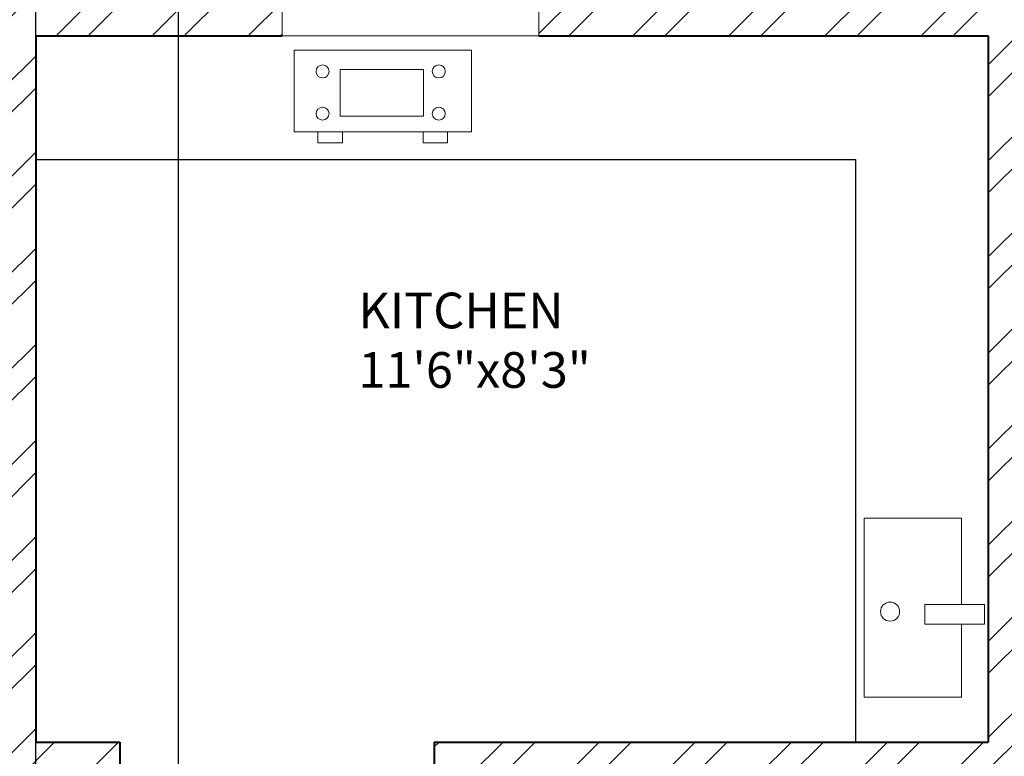
# Model space of a CAD drawing. Units: inches. Extents: x 1601 to 2297, y 1496 to 2631.
# Tile 55 of 57: x 2033 to 2171, y 2422 to 2526. Entities that reach past the tile are written whole.
import ezdxf

# ---------------------------------------------------------------- set-up
doc = ezdxf.new("R2010")
doc.units = ezdxf.units.IN
for name, color, linetype, lineweight in [('A-ANNO-DIMS', 2, 'Continuous', 18), ('A-AREA-IDEN', 7, 'Continuous', 18), ('A-EQPM', 8, 'Continuous', 18), ('A-FLOR-CASE', 8, 'Continuous', 25), ('A-FLOR-FIXT', 9, 'Continuous', 20), ('A-GLAZ', 161, 'Continuous', 20), ('A-WALL', 7, 'Continuous', 40), ('A-WALL-PATT', 215, 'Continuous', 13)]:
    doc.layers.add(name, color=color, linetype=linetype, lineweight=lineweight)
doc.styles.get("Standard").update_dxf_attribs({"font": 'arial.ttf'})
doc.dimstyles.get("Standard").update_dxf_attribs({"dimtxt": 0.18, "dimasz": 0.18, "dimexe": 0.18, "dimexo": 0.0625, "dimgap": 0.09, "dimtad": 0, "dimtih": 1, "dimtoh": 1, "dimdec": 4, "dimzin": 0, "dimdsep": 46, "dimtxsty": 'Standard', "dimcen": 0.09, "dimadec": 0, "dimazin": 0, "dimtfac": 1, "dimtdec": 4, "dimtofl": 0, "dimtmove": 0, "dimatfit": 3, "dimfxl": 1, "dimtolj": 1, "dimtzin": 0, "dimarcsym": 0})

# ---------------------------------------------------------------- blocks, each defined once
blk = doc.blocks.new('COOKTOP-4-BURNER')
for points in [[(0, 12.95), (24.89, 12.95), (24.89, 1.51), (0, 1.51)], [(6.45, 10.25), (18.15, 10.25), (18.15, 3.74), (6.45, 3.74)], [(3.35, 1.51), (6.77, 1.51), (6.77, 0), (3.35, 0)], [(18.09, 1.51), (21.52, 1.51), (21.52, 0), (18.09, 0)], [(18.09, 1.51), (21.52, 1.51), (21.52, 0), (18.09, 0)]]:
    blk.add_lwpolyline(points, close=True)
for centre in [(4, 9.99), (20.29, 9.99), (4, 4.07), (20.29, 4.07)]:
    blk.add_circle(centre, 0.91)
blk = doc.blocks.new('SINK-KITCHEN')
blk.add_lwpolyline([(13.62, 10.25), (13.62, 0), (0, 0), (0, 25.08), (13.62, 25.08), (13.62, 13.01)])
blk.add_lwpolyline([(8.47, 13.01), (16.82, 13.01), (16.82, 10.25), (8.47, 10.25)], close=True)
blk.add_circle((3.61, 11.99), 1.34)
blk = doc.blocks.new('*D40')
at = {"layer": 'A-ANNO-DIMS', "color": 0, "lineweight": -2, "transparency": 16777216}
for p, q in [((2035.54, 1986.39), (2035.54, 2581.06)), ((2035.72, 2580.88), (2045.08, 2580.88)), ((2055.37, 2580.88), (2046.01, 2580.88)), ((2055.55, 1986.39), (2055.55, 2581.06))]:
    blk.add_line(p, q, dxfattribs=at)
at = {"layer": 'A-ANNO-DIMS', "color": 0, "transparency": 16777216}
for points in [[(2035.72, 2580.91), (2035.72, 2580.85), (2035.54, 2580.88)], [(2055.37, 2580.91), (2055.37, 2580.85), (2055.55, 2580.88)]]:
    blk.add_solid(points, dxfattribs=at)
at = {"layer": 'Defpoints', "color": 0, "transparency": 16777216}
for p in [(2055.55, 2580.88), (2035.54, 1986.33), (2055.55, 1986.33)]:
    blk.add_point(p, dxfattribs=at)
at = {"layer": 'A-ANNO-DIMS', "color": 0, "transparency": 16777216, "insert": (2045.54, 2580.88), "char_height": 0.18, "attachment_point": 5}
blk.add_mtext('\\A1;20.014', dxfattribs=at)

msp = doc.modelspace()

# ---------------------------------------------------------------- hatches: boundary and pattern name
at = {"layer": 'A-WALL-PATT'}
h = msp.add_hatch(dxfattribs=at)
h.set_pattern_fill('ANSI32', color=256)
h.paths.add_polyline_path([(1842.0336, 2528.0767), (1842.0336, 2532.3254), (1686.0373, 2532.3254), (1686.0373, 2492.9493), (1695.0373, 2492.9493), (1695.0373, 2523.3254), (1827.0373, 2523.3254), (1827.0373, 2416.8254), (1834.6225, 2416.8254), (1834.6225, 2419.0754), (1834.6225, 2421.3254), (1831.5373, 2421.3254), (1831.5373, 2523.3254), (1842.0336, 2523.3254)])
h.paths.add_polyline_path([(1695.0373, 2432.9493), (1686.0373, 2432.9493), (1686.0373, 2325.989), (1695.0373, 2325.989), (1695.0373, 2347.8254), (1827.0373, 2347.8254), (1827.0373, 2287.8254), (1823.2991, 2287.8254), (1823.2991, 2283.3254), (1847.9422, 2283.3254), (1847.9422, 2285.5754), (1847.9422, 2287.8254), (1831.5373, 2287.8254), (1831.5373, 2347.8254), (1846.9946, 2347.8254), (1846.9946, 2350.0754), (1846.9946, 2352.3254), (1695.0373, 2352.3254)])
h.paths.add_polyline_path([(1807.1169, 1573.5395), (2055.0405, 1573.5395), (2055.0405, 1610.6322), (1807.1169, 1610.6322)], flags=9)
h.paths.add_polyline_path([(1841.1631, 1712.7967), (1870.3957, 1712.7967), (1870.3957, 1731.454), (1841.1631, 1731.454)], flags=9)
h.paths.add_polyline_path([(2144.3862, 1772.185), (2191.0233, 1772.185), (2191.0233, 1790.8423), (2144.3862, 1790.8423)], flags=9)
h.paths.add_polyline_path([(2143.0128, 1827.3312), (2177.9958, 1827.3312), (2177.9958, 1845.9886), (2143.0128, 1845.9886)], flags=9)
h.paths.add_polyline_path([(2041.2439, 1833.5691), (2070.8516, 1833.5691), (2070.8516, 1852.2264), (2041.2439, 1852.2264)], flags=9)
h.paths.add_polyline_path([(2097.2791, 1947.0598), (2134.2061, 1947.0598), (2134.2061, 1965.7171), (2097.2791, 1965.7171)], flags=9)
h.paths.add_polyline_path([(2214.995, 1904.3124), (2214.995, 1942.2899), (2196.3376, 1942.2899), (2196.3376, 1904.3124)], flags=9)
h.paths.add_polyline_path([(2186.6284, 2043.8031), (2219.7935, 2043.8031), (2219.7935, 2062.4605), (2186.6284, 2062.4605)], flags=9)
h.paths.add_polyline_path([(2064.0877, 2031.616), (2097.4949, 2031.616), (2097.4949, 2050.2734), (2064.0877, 2050.2734)], flags=9)
h.paths.add_polyline_path([(1973.1349, 1986.0688), (2008.4009, 1986.0688), (2008.4009, 2004.7261), (1973.1349, 2004.7261)], flags=9)
h.paths.add_polyline_path([(1976.3676, 2106.9635), (2005.7469, 2106.9635), (2005.7469, 2125.6209), (1976.3676, 2125.6209)], flags=9)
h.paths.add_polyline_path([(1991.7852, 2180.4863), (2027.0513, 2180.4863), (2027.0513, 2199.1437), (1991.7852, 2199.1437)], flags=9)
h.paths.add_polyline_path([(2106.1801, 2187.9359), (2152.2101, 2187.9359), (2152.2101, 2206.5932), (2106.1801, 2206.5932)], flags=9)
h.paths.add_polyline_path([(2148.6686, 2262.2542), (2182.318, 2262.2542), (2182.318, 2280.9115), (2148.6686, 2280.9115)], flags=9)
h.paths.add_polyline_path([(2041.6327, 2252.8147), (2071.2405, 2252.8147), (2071.2405, 2271.4721), (2041.6327, 2271.4721)], flags=9)
h.paths.add_polyline_path([(2063.9734, 2375.4265), (2100.9004, 2375.4265), (2100.9004, 2394.0839), (2063.9734, 2394.0839)], flags=9)
h.paths.add_polyline_path([(2216.4955, 2330.9748), (2216.4955, 2370.2654), (2197.8381, 2370.2654), (2197.8381, 2330.9748)], flags=9)
h.paths.add_polyline_path([(2179.1416, 2485.8687), (2212.3067, 2485.8687), (2212.3067, 2504.5261), (2179.1416, 2504.5261)], flags=9)
h.paths.add_polyline_path([(2078.7442, 2471.1516), (2112.1514, 2471.1516), (2112.1514, 2489.809), (2078.7442, 2489.809)], flags=9)
h.paths.add_polyline_path([(1915.9631, 2329.4668), (1952.8902, 2329.4668), (1952.8902, 2348.1241), (1915.9631, 2348.1241)], flags=9)
h.paths.add_polyline_path([(1904.3189, 2499.6709), (1940.4512, 2499.6709), (1940.4512, 2518.3282), (1904.3189, 2518.3282)], flags=9)
h.paths.add_polyline_path([(1892.3665, 2100.4595), (1925.6374, 2100.4595), (1925.6374, 2119.1169), (1892.3665, 2119.1169)], flags=9)
h.paths.add_polyline_path([(1909.2984, 1805.9631), (1946.2254, 1805.9631), (1946.2254, 1824.6205), (1909.2984, 1824.6205)], flags=9)
h.paths.add_polyline_path([(1934.6056, 1658.616), (1970.738, 1658.616), (1970.738, 1677.2733), (1934.6056, 1677.2733)], flags=9)
h.paths.add_polyline_path([(1711.2052, 1789.8902), (1750.0456, 1789.8902), (1750.0456, 1808.5476), (1711.2052, 1808.5476)], flags=9)
h.paths.add_polyline_path([(1742.7874, 1854.6743), (1771.9449, 1854.6743), (1771.9449, 1873.3317), (1742.7874, 1873.3317)], flags=9)
h.paths.add_polyline_path([(1807.3592, 1997.7912), (1850.1116, 1997.7912), (1850.1116, 2016.4486), (1807.3592, 2016.4486)], flags=9)
h.paths.add_polyline_path([(1717.4579, 2237.7844), (1760.2103, 2237.7844), (1760.2103, 2256.4417), (1717.4579, 2256.4417)], flags=9)
h.paths.add_polyline_path([(1780.9285, 2324.0623), (1810.086, 2324.0623), (1810.086, 2342.7197), (1780.9285, 2342.7197)], flags=25)
h.paths.add_polyline_path([(1837.696, 2449.2024), (1866.9286, 2449.2024), (1866.9286, 2467.8598), (1837.696, 2467.8598)], flags=9)
h.paths.add_polyline_path([(1712.7752, 2484.9404), (1751.6156, 2484.9404), (1751.6156, 2503.5977), (1712.7752, 2503.5977)], flags=25)
h = msp.add_hatch(dxfattribs=at)
h.set_pattern_fill('ANSI32', color=256)
h.paths.add_polyline_path([(2230.5373, 2532.3254), (2106.0595, 2532.3254), (2106.0595, 2523.3254), (2169.0373, 2523.3254), (2169.0373, 2424.3254), (2091.3989, 2424.3254), (2091.3989, 2419.8254), (2169.0373, 2419.8254), (2169.0373, 2408.1385), (2178.0373, 2408.1385), (2178.0373, 2419.8254), (2181.0581, 2419.8254), (2181.0581, 2422.0754), (2181.0581, 2424.3254), (2178.0373, 2424.3254), (2178.0373, 2523.3254), (2226.0373, 2523.3254), (2226.0373, 2424.3254), (2206.6251, 2424.3254), (2206.6251, 2419.8254), (2226.0373, 2419.8254), (2226.0373, 2299.8254), (2226.0373, 2295.3254), (2178.0373, 2295.3254), (2178.0373, 2312.1385), (2169.0373, 2312.1385), (2169.0373, 2295.3254), (2130.0373, 2295.3254), (2130.0373, 2279.1364), (2128.0593, 2279.1364), (2128.0593, 2274.6364), (2130.0373, 2274.6364), (2130.0373, 2260.7505), (2134.5373, 2260.7505), (2134.5373, 2290.8254), (2226.0373, 2290.8254), (2226.0373, 2279.2475), (2230.5373, 2279.2475), (2230.5373, 2347.8254)])
h.paths.add_polyline_path([(2070.0595, 2532.3254), (2031.0373, 2532.3254), (2031.0373, 2466.3254), (2003.9878, 2466.3254), (2003.9878, 2457.3254), (2031.0373, 2457.3254), (2031.0373, 2419.8254), (2031.0373, 2373.1914), (2035.5373, 2373.1914), (2035.5373, 2419.8254), (2047.3393, 2419.8254), (2047.3393, 2424.3254), (2035.5373, 2424.3254), (2035.5373, 2523.3254), (2070.0595, 2523.3254), (2070.0595, 2527.8254)])
h.paths.add_polyline_path([(1893.0373, 2532.3254), (1866.0336, 2532.3254), (1866.0336, 2523.3254), (1888.5373, 2523.3254), (1888.5373, 2347.8254), (1893.0373, 2347.8254), (1893.0373, 2457.3254), (1907.9878, 2457.3254), (1907.9878, 2466.3254), (1893.0373, 2466.3254)])
h = msp.add_hatch(dxfattribs=at)
h.set_pattern_fill('ANSI32', color=256)
h.paths.add_polyline_path([(1973.9371, 2211.3254), (1893.0373, 2211.3254), (1893.0373, 2287.8254), (1884.6167, 2287.8254), (1884.6167, 2285.5754), (1884.6167, 2283.3254), (1888.5373, 2283.3254), (1888.5373, 2145.3254), (1695.0373, 2145.3254), (1695.0373, 2173.8724), (1690.5373, 2173.8724), (1686.0373, 2173.8724), (1686.0373, 2136.3254), (1722.5687, 2136.3254), (1722.5687, 2117.4352), (1731.5687, 2117.4352), (1731.5687, 2136.3254), (1893.0373, 2136.3254), (1893.0373, 2202.3254), (1959.0373, 2202.3254), (1959.0373, 2182.1303), (1968.0373, 2182.1303), (1968.0373, 2202.3254), (1973.9371, 2202.3254)])
h.paths.add_polyline_path([(2094.0373, 2274.6364), (2096.4294, 2274.6364), (2096.4294, 2276.8864), (2096.4294, 2279.1364), (2094.0373, 2279.1364), (2094.0373, 2290.8254), (2094.0373, 2295.3254), (2089.5373, 2295.3254), (2089.5373, 2230.8254), (2035.5373, 2230.8254), (2035.5373, 2299.8254), (2031.0373, 2299.8254), (2031.0373, 2211.3254), (2023.0065, 2211.3254), (2023.0065, 2202.3254), (2031.0373, 2202.3254), (2031.0373, 2140.8254), (1968.0373, 2140.8254), (1968.0373, 2145.9106), (1963.5373, 2145.9106), (1959.0373, 2145.9106), (1959.0373, 2116.839), (1963.5373, 2116.839), (1968.0373, 2116.839), (1968.0373, 2131.8254), (2031.0373, 2131.8254), (2031.0373, 2094.3254), (2031.0373, 2085.3254), (2031.0373, 2056.8254), (1968.0373, 2056.8254), (1968.0373, 2070.4947), (1963.5373, 2070.4947), (1959.0373, 2070.4947), (1959.0373, 2040.3029), (1968.0373, 2040.3029), (1968.0373, 2047.8254), (2031.0373, 2047.8254), (2031.0373, 1983.3254), (2031.0373, 1978.8254), (2021.1979, 1978.8254), (2021.1979, 1974.3254), (2031.0373, 1974.3254), (2031.0373, 1954.3528), (2035.5373, 1954.3528), (2035.5373, 1974.3254), (2035.5373, 1981.8254), (2055.5513, 1981.8254), (2055.5513, 1986.3254), (2035.5373, 1986.3254), (2035.5373, 2047.8254), (2040.0373, 2047.8254), (2040.0373, 2085.3254), (2040.0373, 2094.3254), (2040.0373, 2140.8254), (2035.5373, 2140.8254), (2035.5373, 2226.3254), (2089.5373, 2226.3254), (2094.0373, 2226.3254)])
h.paths.add_polyline_path([(2226.0373, 2230.8254), (2134.5373, 2230.8254), (2134.5373, 2233.5437), (2130.0373, 2233.5437), (2130.0373, 2226.3254), (2134.5373, 2226.3254), (2226.0373, 2226.3254)])
h.paths.add_polyline_path([(1807.1169, 1573.5395), (2055.0405, 1573.5395), (2055.0405, 1610.6322), (1807.1169, 1610.6322)], flags=9)
h.paths.add_polyline_path([(1841.1631, 1712.7967), (1870.3957, 1712.7967), (1870.3957, 1731.454), (1841.1631, 1731.454)], flags=9)
h.paths.add_polyline_path([(2144.3862, 1772.185), (2191.0233, 1772.185), (2191.0233, 1790.8423), (2144.3862, 1790.8423)], flags=9)
h.paths.add_polyline_path([(2143.0128, 1827.3312), (2177.9958, 1827.3312), (2177.9958, 1845.9886), (2143.0128, 1845.9886)], flags=9)
h.paths.add_polyline_path([(2041.2439, 1833.5691), (2070.8516, 1833.5691), (2070.8516, 1852.2264), (2041.2439, 1852.2264)], flags=9)
h.paths.add_polyline_path([(2097.2791, 1947.0598), (2134.2061, 1947.0598), (2134.2061, 1965.7171), (2097.2791, 1965.7171)], flags=9)
h.paths.add_polyline_path([(2214.995, 1904.3124), (2214.995, 1942.2899), (2196.3376, 1942.2899), (2196.3376, 1904.3124)], flags=9)
h.paths.add_polyline_path([(2186.6284, 2043.8031), (2219.7935, 2043.8031), (2219.7935, 2062.4605), (2186.6284, 2062.4605)], flags=9)
h.paths.add_polyline_path([(2064.0877, 2031.616), (2097.4949, 2031.616), (2097.4949, 2050.2734), (2064.0877, 2050.2734)], flags=9)
h.paths.add_polyline_path([(1973.1349, 1986.0688), (2008.4009, 1986.0688), (2008.4009, 2004.7261), (1973.1349, 2004.7261)], flags=25)
h.paths.add_polyline_path([(1976.3676, 2106.9635), (2005.7469, 2106.9635), (2005.7469, 2125.6209), (1976.3676, 2125.6209)], flags=25)
h.paths.add_polyline_path([(1991.7852, 2180.4863), (2027.0513, 2180.4863), (2027.0513, 2199.1437), (1991.7852, 2199.1437)], flags=25)
h.paths.add_polyline_path([(2106.1801, 2187.9359), (2152.2101, 2187.9359), (2152.2101, 2206.5932), (2106.1801, 2206.5932)], flags=9)
h.paths.add_polyline_path([(2148.6686, 2262.2542), (2182.318, 2262.2542), (2182.318, 2280.9115), (2148.6686, 2280.9115)], flags=9)
h.paths.add_polyline_path([(2041.6327, 2252.8147), (2071.2405, 2252.8147), (2071.2405, 2271.4721), (2041.6327, 2271.4721)], flags=25)
h.paths.add_polyline_path([(2063.9734, 2375.4265), (2100.9004, 2375.4265), (2100.9004, 2394.0839), (2063.9734, 2394.0839)], flags=9)
h.paths.add_polyline_path([(2216.4955, 2330.9748), (2216.4955, 2370.2654), (2197.8381, 2370.2654), (2197.8381, 2330.9748)], flags=9)
h.paths.add_polyline_path([(2179.1416, 2485.8687), (2212.3067, 2485.8687), (2212.3067, 2504.5261), (2179.1416, 2504.5261)], flags=9)
h.paths.add_polyline_path([(2078.7442, 2471.1516), (2112.1514, 2471.1516), (2112.1514, 2489.809), (2078.7442, 2489.809)], flags=9)
h.paths.add_polyline_path([(1915.9631, 2329.4668), (1952.8902, 2329.4668), (1952.8902, 2348.1241), (1915.9631, 2348.1241)], flags=9)
h.paths.add_polyline_path([(1904.3189, 2499.6709), (1940.4512, 2499.6709), (1940.4512, 2518.3282), (1904.3189, 2518.3282)], flags=9)
h.paths.add_polyline_path([(1892.3665, 2100.4595), (1925.6374, 2100.4595), (1925.6374, 2119.1169), (1892.3665, 2119.1169)], flags=9)
h.paths.add_polyline_path([(1909.2984, 1805.9631), (1946.2254, 1805.9631), (1946.2254, 1824.6205), (1909.2984, 1824.6205)], flags=9)
h.paths.add_polyline_path([(1934.6056, 1658.616), (1970.738, 1658.616), (1970.738, 1677.2733), (1934.6056, 1677.2733)], flags=9)
h.paths.add_polyline_path([(1711.2052, 1789.8902), (1750.0456, 1789.8902), (1750.0456, 1808.5476), (1711.2052, 1808.5476)], flags=9)
h.paths.add_polyline_path([(1742.7874, 1854.6743), (1771.9449, 1854.6743), (1771.9449, 1873.3317), (1742.7874, 1873.3317)], flags=9)
h.paths.add_polyline_path([(1807.3592, 1997.7912), (1850.1116, 1997.7912), (1850.1116, 2016.4486), (1807.3592, 2016.4486)], flags=9)
h.paths.add_polyline_path([(1717.4579, 2237.7844), (1760.2103, 2237.7844), (1760.2103, 2256.4417), (1717.4579, 2256.4417)], flags=25)
h.paths.add_polyline_path([(1780.9285, 2324.0623), (1810.086, 2324.0623), (1810.086, 2342.7197), (1780.9285, 2342.7197)], flags=9)
h.paths.add_polyline_path([(1837.696, 2449.2024), (1866.9286, 2449.2024), (1866.9286, 2467.8598), (1837.696, 2467.8598)], flags=9)
h.paths.add_polyline_path([(1712.7752, 2484.9404), (1751.6156, 2484.9404), (1751.6156, 2503.5977), (1712.7752, 2503.5977)], flags=9)
h = msp.add_hatch(dxfattribs=at)
h.set_pattern_fill('ANSI32', color=256)
h.paths.add_polyline_path([(2230.5373, 1861.8254), (2182.5373, 1861.8254), (2182.5373, 1885.3637), (2178.0373, 1885.3637), (2178.0373, 1861.8254), (2166.0373, 1861.8254), (2134.5373, 1861.8254), (2130.0373, 1861.8254), (2130.0373, 1841.4682), (2126.8833, 1841.4682), (2126.8833, 1836.9682), (2130.0373, 1836.9682), (2130.0373, 1822.7302), (2134.5373, 1822.7302), (2134.5373, 1857.3254), (2166.0373, 1857.3254), (2226.0373, 1857.3254), (2226.0373, 1846.1155), (2230.5373, 1846.1155)])
h.paths.add_polyline_path([(2226.0373, 1797.3254), (2134.5373, 1797.3254), (2134.5373, 1800.6636), (2132.2873, 1800.6636), (2130.0373, 1800.6636), (2130.0373, 1797.3254), (2130.0373, 1792.8254), (2167.7264, 1792.8254), (2226.0373, 1792.8254)])
h.paths.add_polyline_path([(2230.5373, 1822.1155), (2226.0373, 1822.1155), (2226.0373, 1760.8563), (2230.5373, 1760.8563)])
h.paths.add_polyline_path([(2230.5373, 1700.8563), (2226.0373, 1700.8563), (2226.0373, 1644.3254), (2140.2517, 1644.3254), (2140.2517, 1635.3254), (2230.5373, 1635.3254)])
h.paths.add_polyline_path([(2080.2517, 1639.8254), (2080.2517, 1644.3254), (2035.5373, 1644.3254), (2035.5373, 1792.8254), (2094.0373, 1792.8254), (2094.0373, 1797.3254), (2094.0373, 1836.9682), (2097.1057, 1836.9682), (2097.1057, 1839.2182), (2097.1057, 1841.4682), (2094.0373, 1841.4682), (2094.0373, 1862.2276), (2089.5373, 1862.2276), (2089.5373, 1797.3254), (2035.5373, 1797.3254), (2035.5373, 1857.3254), (2035.5373, 1885.0916), (2031.0373, 1885.0916), (2031.0373, 1710.3254), (2012.329, 1710.3254), (2012.329, 1701.3254), (2031.0373, 1701.3254), (2031.0373, 1644.3254), (2031.0373, 1635.3254), (2080.2517, 1635.3254)])
h.paths.add_polyline_path([(1836.0373, 1653.2033), (1842.6171, 1653.2033), (1842.6171, 1657.7033), (1842.6171, 1662.2033), (1831.5373, 1662.2033), (1831.5373, 1764.2033), (1835.3881, 1764.2033), (1835.3881, 1766.4533), (1835.3881, 1768.7033), (1831.5373, 1768.7033), (1827.0373, 1768.7033), (1827.0373, 1662.2033), (1827.0373, 1635.3254), (1836.0373, 1635.3254)])
h.paths.add_polyline_path([(1893.0373, 1701.3254), (1907.193, 1701.3254), (1907.193, 1705.8254), (1907.193, 1710.3254), (1893.0373, 1710.3254), (1893.0373, 1819.8254), (1882.6444, 1819.8254), (1882.6444, 1817.5754), (1882.6444, 1815.3254), (1888.5373, 1815.3254), (1888.5373, 1662.2033), (1884.0373, 1662.2033), (1866.6171, 1662.2033), (1866.6171, 1653.2033), (1882.391, 1653.2033), (1884.0373, 1653.2033), (1884.0373, 1635.3254), (1893.0373, 1635.3254)])
h.paths.add_polyline_path([(1739.3335, 1639.8254), (1739.3335, 1644.3254), (1695.0373, 1644.3254), (1695.0373, 1702.0135), (1690.5373, 1702.0135), (1686.0373, 1702.0135), (1686.0373, 1635.3254), (1739.3335, 1635.3254)])
h.paths.add_polyline_path([(1827.0373, 1644.3254), (1799.3335, 1644.3254), (1799.3335, 1635.3254), (1827.0373, 1635.3254)])
h.paths.add_polyline_path([(1695.0373, 1815.3254), (1849.2759, 1815.3254), (1849.2759, 1819.8254), (1807.5373, 1819.8254), (1807.5373, 1879.8254), (1851.1533, 1879.8254), (1851.1533, 1882.0754), (1851.1533, 1884.3254), (1799.3405, 1884.3254), (1799.3405, 1882.0754), (1799.3405, 1879.8254), (1803.0373, 1879.8254), (1803.0373, 1819.8254), (1695.0373, 1819.8254), (1695.0373, 1835.0458), (1690.5373, 1835.0458), (1686.0373, 1835.0458), (1686.0373, 1766.1753), (1695.0373, 1766.1753)])
h.paths.add_polyline_path([(1775.8157, 1884.3254), (1695.0373, 1884.3254), (1695.0373, 1912.9526), (1690.5373, 1912.9526), (1686.0373, 1912.9526), (1686.0373, 1859.0458), (1695.0373, 1859.0458), (1695.0373, 1879.8254), (1775.8157, 1879.8254)])
h.paths.add_polyline_path([(1893.0373, 2031.3254), (1731.5687, 2031.3254), (1731.5687, 2057.4352), (1722.5687, 2057.4352), (1722.5687, 2031.3254), (1686.0373, 2031.3254), (1686.0373, 1972.9526), (1695.0373, 1972.9526), (1695.0373, 2022.3254), (1888.5373, 2022.3254), (1888.5373, 1884.3254), (1883.4996, 1884.3254), (1883.4996, 1879.8254), (1893.0373, 1879.8254), (1893.0373, 1974.3254), (1976.6199, 1974.3254), (1976.6199, 1978.8254), (1968.0373, 1978.8254), (1968.0373, 1983.3254), (1968.0373, 2008.4756), (1963.5373, 2008.4756), (1959.0373, 2008.4756), (1959.0373, 1983.3254), (1893.0373, 1983.3254)])
h.paths.add_polyline_path([(2230.5373, 2140.4745), (2226.0373, 2140.4745), (2226.0373, 2094.3254), (2040.0373, 2094.3254), (2040.0373, 2085.3254), (2178.0373, 2085.3254), (2178.0373, 2065.6965), (2182.5373, 2065.6965), (2182.5373, 2085.3254), (2226.0373, 2085.3254), (2226.0373, 1986.3254), (2211.2679, 1986.3254), (2211.2679, 1981.8254), (2230.5373, 1981.8254)])
h.paths.add_polyline_path([(2187.6292, 1986.3254), (2182.5373, 1986.3254), (2182.5373, 2029.6965), (2178.0373, 2029.6965), (2178.0373, 1986.3254), (2099.05, 1986.3254), (2099.05, 1981.8254), (2178.0373, 1981.8254), (2178.0373, 1969.3637), (2182.5373, 1969.3637), (2182.5373, 1981.8254), (2187.6292, 1981.8254), (2187.6292, 1984.0754)])
h.paths.add_polyline_path([(1807.1169, 1573.5395), (2055.0405, 1573.5395), (2055.0405, 1610.6322), (1807.1169, 1610.6322)], flags=9)
h.paths.add_polyline_path([(1841.1631, 1712.7967), (1870.3957, 1712.7967), (1870.3957, 1731.454), (1841.1631, 1731.454)], flags=9)
h.paths.add_polyline_path([(2144.3862, 1772.185), (2191.0233, 1772.185), (2191.0233, 1790.8423), (2144.3862, 1790.8423)], flags=9)
h.paths.add_polyline_path([(2143.0128, 1827.3312), (2177.9958, 1827.3312), (2177.9958, 1845.9886), (2143.0128, 1845.9886)], flags=25)
h.paths.add_polyline_path([(2041.2439, 1833.5691), (2070.8516, 1833.5691), (2070.8516, 1852.2264), (2041.2439, 1852.2264)], flags=25)
h.paths.add_polyline_path([(2097.2791, 1947.0598), (2134.2061, 1947.0598), (2134.2061, 1965.7171), (2097.2791, 1965.7171)], flags=9)
h.paths.add_polyline_path([(2214.995, 1904.3124), (2214.995, 1942.2899), (2196.3376, 1942.2899), (2196.3376, 1904.3124)], flags=9)
h.paths.add_polyline_path([(2186.6284, 2043.8031), (2219.7935, 2043.8031), (2219.7935, 2062.4605), (2186.6284, 2062.4605)], flags=25)
h.paths.add_polyline_path([(2064.0877, 2031.616), (2097.4949, 2031.616), (2097.4949, 2050.2734), (2064.0877, 2050.2734)], flags=25)
h.paths.add_polyline_path([(1973.1349, 1986.0688), (2008.4009, 1986.0688), (2008.4009, 2004.7261), (1973.1349, 2004.7261)], flags=9)
h.paths.add_polyline_path([(1976.3676, 2106.9635), (2005.7469, 2106.9635), (2005.7469, 2125.6209), (1976.3676, 2125.6209)], flags=9)
h.paths.add_polyline_path([(1991.7852, 2180.4863), (2027.0513, 2180.4863), (2027.0513, 2199.1437), (1991.7852, 2199.1437)], flags=9)
h.paths.add_polyline_path([(2106.1801, 2187.9359), (2152.2101, 2187.9359), (2152.2101, 2206.5932), (2106.1801, 2206.5932)], flags=9)
h.paths.add_polyline_path([(2148.6686, 2262.2542), (2182.318, 2262.2542), (2182.318, 2280.9115), (2148.6686, 2280.9115)], flags=9)
h.paths.add_polyline_path([(2041.6327, 2252.8147), (2071.2405, 2252.8147), (2071.2405, 2271.4721), (2041.6327, 2271.4721)], flags=9)
h.paths.add_polyline_path([(2063.9734, 2375.4265), (2100.9004, 2375.4265), (2100.9004, 2394.0839), (2063.9734, 2394.0839)], flags=9)
h.paths.add_polyline_path([(2216.4955, 2330.9748), (2216.4955, 2370.2654), (2197.8381, 2370.2654), (2197.8381, 2330.9748)], flags=9)
h.paths.add_polyline_path([(2179.1416, 2485.8687), (2212.3067, 2485.8687), (2212.3067, 2504.5261), (2179.1416, 2504.5261)], flags=9)
h.paths.add_polyline_path([(2078.7442, 2471.1516), (2112.1514, 2471.1516), (2112.1514, 2489.809), (2078.7442, 2489.809)], flags=9)
h.paths.add_polyline_path([(1915.9631, 2329.4668), (1952.8902, 2329.4668), (1952.8902, 2348.1241), (1915.9631, 2348.1241)], flags=9)
h.paths.add_polyline_path([(1904.3189, 2499.6709), (1940.4512, 2499.6709), (1940.4512, 2518.3282), (1904.3189, 2518.3282)], flags=9)
h.paths.add_polyline_path([(1892.3665, 2100.4595), (1925.6374, 2100.4595), (1925.6374, 2119.1169), (1892.3665, 2119.1169)], flags=9)
h.paths.add_polyline_path([(1909.2984, 1805.9631), (1946.2254, 1805.9631), (1946.2254, 1824.6205), (1909.2984, 1824.6205)], flags=9)
h.paths.add_polyline_path([(1934.6056, 1658.616), (1970.738, 1658.616), (1970.738, 1677.2733), (1934.6056, 1677.2733)], flags=9)
h.paths.add_polyline_path([(1711.2052, 1789.8902), (1750.0456, 1789.8902), (1750.0456, 1808.5476), (1711.2052, 1808.5476)], flags=25)
h.paths.add_polyline_path([(1742.7874, 1854.6743), (1771.9449, 1854.6743), (1771.9449, 1873.3317), (1742.7874, 1873.3317)], flags=25)
h.paths.add_polyline_path([(1807.3592, 1997.7912), (1850.1116, 1997.7912), (1850.1116, 2016.4486), (1807.3592, 2016.4486)], flags=25)
h.paths.add_polyline_path([(1717.4579, 2237.7844), (1760.2103, 2237.7844), (1760.2103, 2256.4417), (1717.4579, 2256.4417)], flags=9)
h.paths.add_polyline_path([(1780.9285, 2324.0623), (1810.086, 2324.0623), (1810.086, 2342.7197), (1780.9285, 2342.7197)], flags=9)
h.paths.add_polyline_path([(1837.696, 2449.2024), (1866.9286, 2449.2024), (1866.9286, 2467.8598), (1837.696, 2467.8598)], flags=9)
h.paths.add_polyline_path([(1712.7752, 2484.9404), (1751.6156, 2484.9404), (1751.6156, 2503.5977), (1712.7752, 2503.5977)], flags=9)

# ---------------------------------------------------------------- linework, layer by layer
at = {"layer": 'A-FLOR-CASE'}
for p, q in [((2035.5373, 2505.9908), (2150.4298, 2505.9908)), ((2150.4298, 2505.9908), (2150.4298, 2424.3254)), ((2150.4298, 2424.3254), (2150.4298, 2424.3254))]:
    msp.add_line(p, q, dxfattribs=at)
at = {"layer": 'A-GLAZ'}
for p, q in [((2070.0595, 2532.3254), (2070.0595, 2523.3254)), ((2106.0595, 2532.3254), (2106.0595, 2523.3254)), ((2070.0595, 2523.3254), (2070.0595, 2527.8254)), ((2106.0595, 2523.3254), (2070.0595, 2523.3254))]:
    msp.add_line(p, q, dxfattribs=at)
at = {"layer": 'A-WALL'}
for p, q in [((2035.5373, 2523.3254), (2035.5373, 2424.3254)), ((2035.5373, 2523.3254), (2070.0595, 2523.3254)), ((2106.0595, 2523.3254), (2169.0373, 2523.3254)), ((2169.0373, 2523.3254), (2169.0373, 2424.3254)), ((2035.5373, 2424.3254), (2047.3393, 2424.3254)), ((2047.3393, 2424.3254), (2047.3393, 2419.8254)), ((2091.3989, 2424.3254), (2091.3989, 2419.8254)), ((2091.3989, 2424.3254), (2169.0373, 2424.3254))]:
    msp.add_line(p, q, dxfattribs=at)

# ---------------------------------------------------------------- block references
at = {"layer": 'A-EQPM'}
msp.add_blockref('COOKTOP-4-BURNER', (2071.739, 2508.335), dxfattribs=at)
at = {"layer": 'A-FLOR-FIXT'}
msp.add_blockref('SINK-KITCHEN', (2151.6687, 2430.6248), dxfattribs=at)

# ---------------------------------------------------------------- texts
at = {"layer": 'A-AREA-IDEN', "insert": (2080.7547, 2487.3209), "char_height": 5, "attachment_point": 1}
msp.add_mtext_dynamic_manual_height_columns('KITCHEN\\P11\'6"x8\'3"', width=82.082486, gutter_width=12.5, heights=[0], dxfattribs=at)

# ---------------------------------------------------------------- dimensions: what is measured, and where the dimension line sits
at = {"layer": 'A-ANNO-DIMS'}
dim = msp.add_linear_dim(base=(2055.5513, 2580.8754), p1=(2035.5373, 1986.3254), p2=(2055.5513, 1986.3254), dimstyle='Standard', override={"dimdec": 3, "dimlfac": 1, "dimrnd": 0, "dimzin": 0, "dimdsep": 46, "dimlunit": 2}, dxfattribs=at)
dim.commit()
dim.dimension.update_dxf_attribs({"geometry": '*D40', "text_midpoint": (2045.5443, 2580.8754)})

doc.saveas('drawing.dxf')
